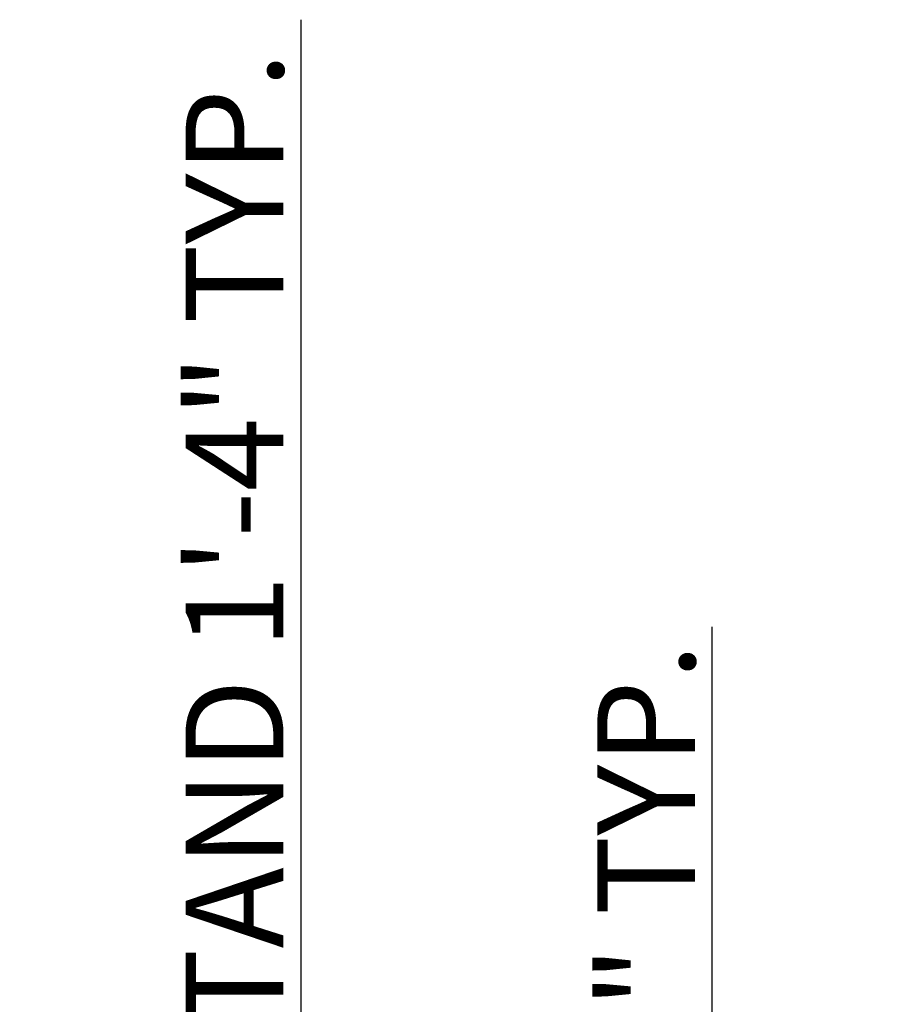
# Model space of a CAD drawing. Units: inches. Extents: x 597 to 1323, y 1833 to 2686.
# Tile 8 of 10: x 740 to 895, y 2509 to 2686. Entities that reach past the tile are written whole.
import ezdxf

# ---------------------------------------------------------------- set-up
doc = ezdxf.new("R2010")
doc.units = ezdxf.units.IN
doc.layers.add('A-ANNO-DIMS', color=2, linetype='Continuous', lineweight=18)
doc.styles.get("Standard").update_dxf_attribs({"font": 'arial.ttf'})
doc.dimstyles.new('ISO-25', dxfattribs={"dimtxt": 17.5, "dimasz": 2.5, "dimexe": 0, "dimexo": 0, "dimtad": 1, "dimdec": 1, "dimlunit": 3, "dimtxsty": 'Standard', "dimblk": 'OPEN90', "dimcen": 2.5, "dimadec": 0, "dimazin": 0, "dimtfac": 1, "dimtdec": 1, "dimtmove": 0, "dimatfit": 3, "dimfxl": 0, "dimfxlon": 1, "dimarcsym": 0})

# ---------------------------------------------------------------- blocks, each defined once
blk = doc.blocks.new('_Open90')
at = {"color": 0, "linetype": 'ByBlock', "lineweight": -2}
for p, q in [((0, 0), (-1, 0)), ((-0.5, 0.5), (0, 0)), ((0, 0), (-0.5, -0.5))]:
    blk.add_line(p, q, dxfattribs=at)
blk = doc.blocks.new('*D33')
at = {"layer": 'A-ANNO-DIMS', "color": 0, "lineweight": -2, "transparency": 16777216}
for p, q in [((790.41, 2410.26), (790.41, 2685.53)), ((790.41, 2396.84), (790.41, 2407.76))]:
    blk.add_line(p, q, dxfattribs=at)
at = {"layer": 'Defpoints', "color": 0, "transparency": 16777216}
for p in [(790.41, 2410.26), (792.8, 2410.26), (792.8, 2394.34)]:
    blk.add_point(p, dxfattribs=at)
at = {"layer": 'A-ANNO-DIMS', "color": 0, "lineweight": -2, "transparency": 16777216, "xscale": 2.5, "yscale": 2.5, "zscale": 2.5}
for p, rotation in [((790.41, 2410.26), 90), ((790.41, 2394.34), 270)]:
    blk.add_blockref('_Open90', p, dxfattribs=dict(at, rotation=rotation))
at = {"layer": 'A-ANNO-DIMS', "color": 0, "transparency": 16777216, "insert": (780.74, 2549.15), "char_height": 17.5, "attachment_point": 5, "rotation": 90}
blk.add_mtext('NIGHTSTAND 1\'-4" TYP.', dxfattribs=at)
blk = doc.blocks.new('*D41')
at = {"layer": 'A-ANNO-DIMS', "color": 0, "lineweight": -2, "transparency": 16777216}
for p, q in [((863.97, 2410.26), (863.97, 2576.96)), ((863.97, 2350.91), (863.97, 2407.76))]:
    blk.add_line(p, q, dxfattribs=at)
at = {"layer": 'Defpoints', "color": 0, "transparency": 16777216}
for p in [(854.69, 2410.26), (863.97, 2410.26), (854.69, 2348.41)]:
    blk.add_point(p, dxfattribs=at)
at = {"layer": 'A-ANNO-DIMS', "color": 0, "lineweight": -2, "transparency": 16777216, "xscale": 2.5, "yscale": 2.5, "zscale": 2.5}
for p, rotation in [((863.97, 2410.26), 90), ((863.97, 2348.41), 270)]:
    blk.add_blockref('_Open90', p, dxfattribs=dict(at, rotation=rotation))
at = {"layer": 'A-ANNO-DIMS', "color": 0, "transparency": 16777216, "insert": (854.41, 2494.86), "char_height": 17.5, "attachment_point": 5, "rotation": 90}
blk.add_mtext('BED 5\'-2" TYP.', dxfattribs=at)

msp = doc.modelspace()

# ---------------------------------------------------------------- dimensions: what is measured, and where the dimension line sits
at = {"layer": 'A-ANNO-DIMS'}
for base, p1, p2, text, picture, middle in [((790.41, 2410.26), (792.8, 2394.34), (792.8, 2410.26), 'NIGHTSTAND <> TYP.', '*D33', (780.74, 2549.15)), ((863.966, 2410.2595), (854.6884, 2348.4086), (854.6884, 2410.2595), 'BED <> TYP.', '*D41', (854.406, 2494.8622))]:
    dim = msp.add_linear_dim(base=base, p1=p1, p2=p2, angle=90, text=text, dimstyle='ISO-25', override={"dimdec": 1, "dimlfac": 1, "dimrnd": 0, "dimzin": 1, "dimdsep": 46, "dimlunit": 4, "dimfrac": 2}, dxfattribs=at)
    dim.commit()
    dim.dimension.update_dxf_attribs({"geometry": picture, "text_midpoint": middle})

doc.saveas('drawing.dxf')
